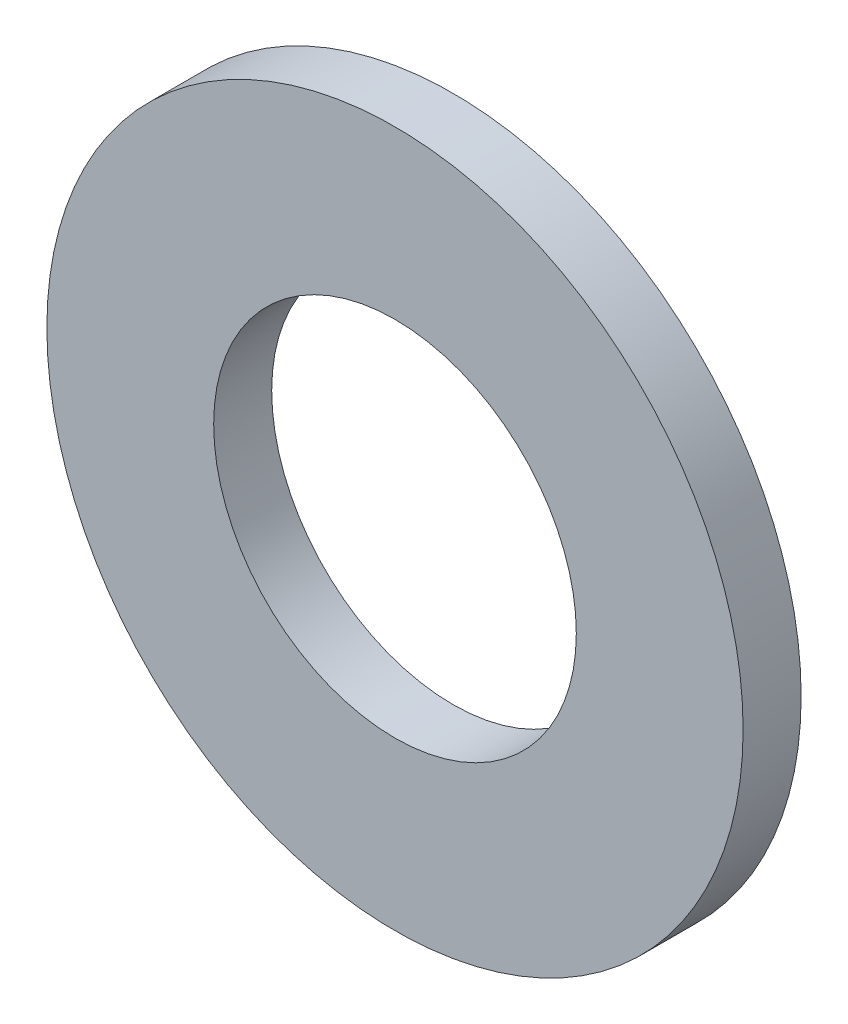
SolidWorks part; units mm, degrees
material "Plain Carbon Steel"
ref_plane "Front Plane" through (0, 0, 0) normal (0, 0, 1) x (1, 0, 0)
ref_plane "Top Plane" through (0, 0, 0) normal (0, 1, 0) x (1, 0, 0)
ref_plane "Right Plane" through (0, 0, 0) normal (1, 0, 0) x (0, 0, -1)
sketch "Washer Profile Ø12 x Ø6.25" plane through (0, 0, 0) normal (0, 0, 1) x (1, 0, 0)
  circle A0 centre (0, 0) radius 3.125
  circle A1 centre (0, 0) radius 6
  dimension "D1" = 6.25
  dimension "D2" = 12
extrude "Washer Body 1mm" add sketch "Washer Profile Ø12 x Ø6.25" along normal mid plane 1
